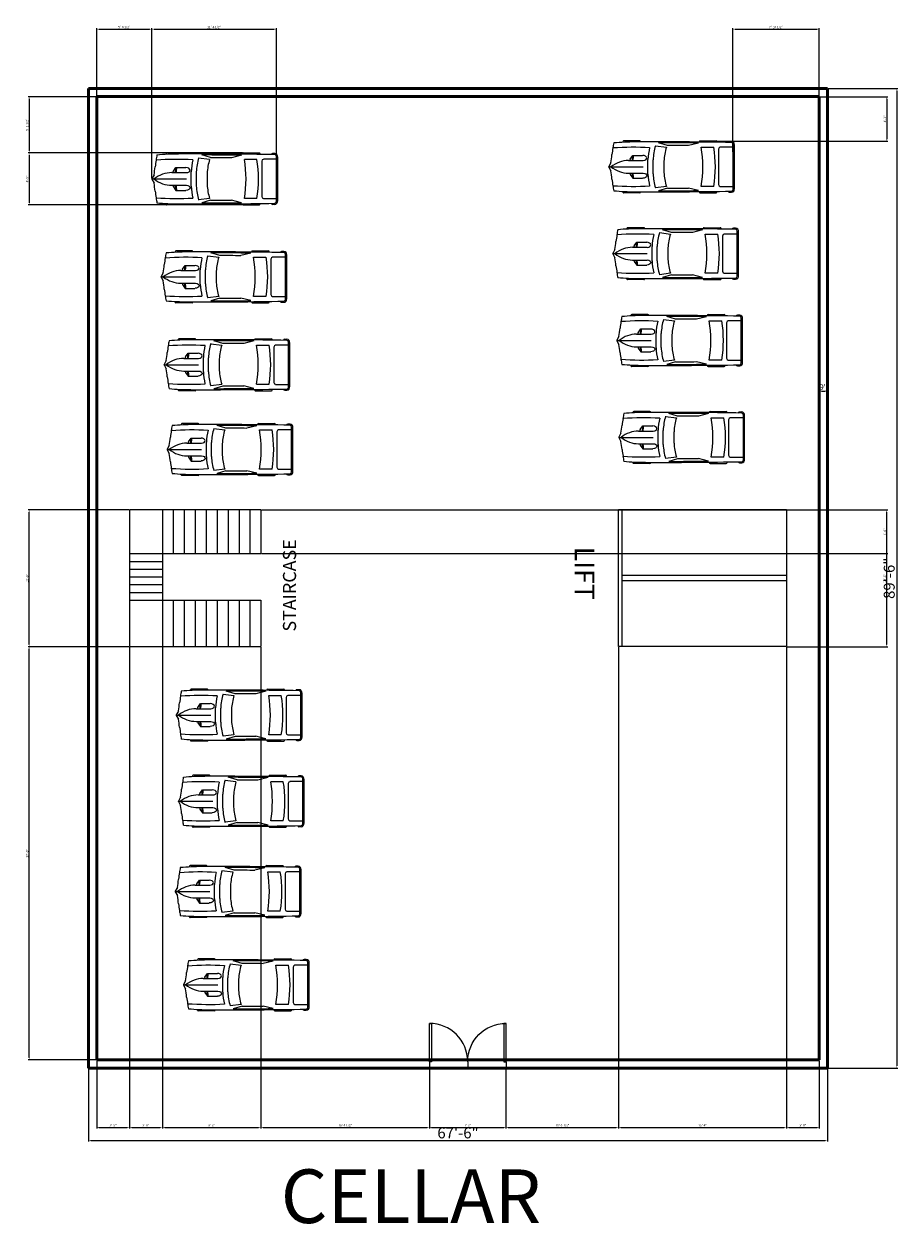
# Model space of a CAD drawing. Units: inches. Extents: x -12550 to 6516, y 1273 to 18700.
# Tile 1 of 19: x 757 to 1715, y 1273 to 2589. Entities that reach past the tile are written whole.
import ezdxf

# ---------------------------------------------------------------- set-up
doc = ezdxf.new("R2010")
doc.units = ezdxf.units.IN
for name, color, linetype, lineweight in [('A-ANNO-DIMS', 2, 'Continuous', 18), ('A-ANNO-TEXT', 7, 'Continuous', 25), ('A-AREA-IDEN', 1, 'Continuous', 18), ('A-DOOR', 5, 'Continuous', 25), ('A-EQPM', 4, 'Continuous', 25), ('A-FLOR-STRS', 6, 'Continuous', 25), ('A-FURN', 8, 'Continuous', 18), ('A-WALL', 7, 'Continuous', 50)]:
    doc.layers.add(name, color=color, linetype=linetype, lineweight=lineweight)
doc.styles.get("Standard").update_dxf_attribs({"font": 'arial.ttf'})
doc.dimstyles.new('ISO-25', dxfattribs={"dimtxt": 2.5, "dimasz": 2.5, "dimexe": 1.25, "dimexo": 0.625, "dimtad": 1, "dimlunit": 4, "dimtxsty": 'Standard', "dimcen": 2.5, "dimadec": 0, "dimazin": 0, "dimtfac": 1, "dimtmove": 0, "dimatfit": 3, "dimfxl": 1, "dimarcsym": 0})

# ---------------------------------------------------------------- blocks, each defined once
blk = doc.blocks.new('*U2')
for p, q in [((0, 0), (0, -5)), ((30, 0), (30, -5))]:
    blk.add_line(p, q)
blk.add_lwpolyline([(0, 0), (0, 30), (1.75, 30), (1.75, 0)], close=True)
blk.add_arc((0, 0), 30, 0, 90)
blk = doc.blocks.new('*D22')
at = {"layer": 'A-ANNO-DIMS', "color": 0, "lineweight": -2, "transparency": 16777216}
for p, q in [((1638, 2518.2), (1714.6, 2518.2)), ((1713.4, 2515.7), (1713.4, 1446.7)), ((1638, 1444.2), (1714.6, 1444.2))]:
    blk.add_line(p, q, dxfattribs=at)
at = {"layer": 'A-ANNO-DIMS', "color": 0, "transparency": 16777216}
for points in [[(1713, 2515.7), (1713.8, 2515.7), (1713.4, 2518.2)], [(1713, 1446.7), (1713.8, 1446.7), (1713.4, 1444.2)]]:
    blk.add_solid(points, dxfattribs=at)
at = {"layer": 'Defpoints', "color": 0, "transparency": 16777216}
for p in [(1637.4, 2518.2), (1637.4, 1444.2), (1713.4, 1444.2)]:
    blk.add_point(p, dxfattribs=at)
at = {"layer": 'A-ANNO-DIMS', "color": 0, "transparency": 16777216, "insert": (1706.6, 1981.2), "char_height": 12, "attachment_point": 5, "rotation": 90}
blk.add_mtext('89\'-6"', dxfattribs=at)
blk = doc.blocks.new('*D23')
at = {"layer": 'A-ANNO-DIMS', "color": 0, "lineweight": -2, "transparency": 16777216}
for p, q in [((827.4, 1443.6), (827.4, 1363.6)), ((1637.4, 1443.6), (1637.4, 1363.6)), ((829.9, 1364.9), (1634.9, 1364.9))]:
    blk.add_line(p, q, dxfattribs=at)
at = {"layer": 'A-ANNO-DIMS', "color": 0, "transparency": 16777216}
for points in [[(829.9, 1365.3), (829.9, 1364.5), (827.4, 1364.9)], [(1634.9, 1365.3), (1634.9, 1364.5), (1637.4, 1364.9)]]:
    blk.add_solid(points, dxfattribs=at)
at = {"layer": 'Defpoints', "color": 0, "transparency": 16777216}
for p in [(827.4, 1444.2), (1637.4, 1444.2), (1637.4, 1364.9)]:
    blk.add_point(p, dxfattribs=at)
at = {"layer": 'A-ANNO-DIMS', "color": 0, "transparency": 16777216, "insert": (1232.4, 1371.6), "char_height": 12, "attachment_point": 5}
blk.add_mtext('67\'-6"', dxfattribs=at)
blk = doc.blocks.new('*D24')
at = {"layer": 'A-ANNO-DIMS', "color": 0, "lineweight": -2, "transparency": 16777216}
for p, q in [((1628.4, 2172.1), (1628.4, 2187.7)), ((1630.9, 2186.4), (1634.9, 2186.4)), ((1637.4, 2172.1), (1637.4, 2187.7))]:
    blk.add_line(p, q, dxfattribs=at)
at = {"layer": 'A-ANNO-DIMS', "color": 0, "transparency": 16777216}
for points in [[(1630.9, 2186.9), (1630.9, 2186), (1628.4, 2186.4)], [(1634.9, 2186.9), (1634.9, 2186), (1637.4, 2186.4)]]:
    blk.add_solid(points, dxfattribs=at)
at = {"layer": 'Defpoints', "color": 0, "transparency": 16777216}
for p in [(1637.4, 2186.4), (1628.4, 2171.4), (1637.4, 2171.4)]:
    blk.add_point(p, dxfattribs=at)
at = {"layer": 'A-ANNO-DIMS', "color": 0, "transparency": 16777216, "insert": (1632.9, 2190.1), "char_height": 6, "attachment_point": 5}
blk.add_mtext('9"', dxfattribs=at)
blk = doc.blocks.new('*U21')
for p, q in [((21.1, 37.4), (21.1, 36.8)), ((46.6, 38.9), (22.4, 38.9)), ((47.8, 37.4), (47.8, 37.4)), ((135.5, 37.1), (135.5, 37.4)), ((136.7, 38.9), (160.9, 38.9)), ((162.1, 37.4), (162.1, 36.8)), ((70, 31.5), (86.4, 29.4)), ((88, 31.9), (74.8, 35.9)), ((134.3, 35.6), (119.3, 31.8)), ((138.4, 29.4), (157.2, 29.4)), ((164.5, 26.4), (164.5, -26.4)), ((186.5, 29.4), (167, 29.4)), ((186.5, -33.5), (186.5, 33.5)), ((188.4, -32.8), (188.4, 32.8)), ((3.3, 6.1), (0.1, 0.4)), ((29.8, 9.5), (51.7, 9.5)), ((32.1, 9.5), (32.1, 11.2)), ((32.3, 11.6), (36.1, 17.2)), ((36.1, 17.2), (50.9, 17.2)), ((58.9, -10.8), (58.9, 10.8)), ((66.6, -10.5), (66.6, 10.5)), ((82.7, 8.5), (82.7, -8.5)), ((186.5, -10.5), (186.5, 10.5)), ((0, 0), (51.7, 0)), ((0.1, -0.4), (3.3, -6.1)), ((29.8, -9.5), (51.7, -9.5)), ((32.1, -9.5), (32.1, -11.2)), ((32.3, -11.6), (36.1, -17.2)), ((36.1, -17.2), (50.9, -17.2)), ((86.4, -29.4), (70, -31.5)), ((88, -31.9), (74.8, -35.9)), ((134.3, -35.6), (119.3, -31.8)), ((157.2, -29.4), (138.4, -29.4)), ((167, -29.4), (186.5, -29.4)), ((21.1, -37.4), (21.1, -36.8)), ((46.6, -38.9), (22.4, -38.9)), ((47.8, -37.4), (47.8, -37.4)), ((135.5, -37.1), (135.5, -37.4)), ((136.7, -38.9), (160.9, -38.9)), ((162.1, -37.4), (162.1, -36.8))]:
    blk.add_line(p, q)
for centre, major_axis, ratio, start_param, end_param in [((41.2, -490.9), (0, 528.2), 0.842304, 0.00281, 0.075598), ((22.4, 37.4), (0, -1.48), 0.842304, 3.141593, 4.712389), ((64.5, -10555.6), (0, 10593), 0.842304, -0.013397, 0.002797), ((46.6, 37.4), (0, 1.48), 0.842304, -1.570796, 0), ((136.7, 37.4), (0, -1.48), 0.842304, 3.141593, 4.712389), ((160.9, 37.4), (0, 1.48), 0.842304, -1.570796, 0), ((180.6, 35.8), (0, 2.22), 0.842304, -0.013017, 1.249894), ((64.5, -10556.4), (0, 10595.3), 0.842304, -0.013397, -0.013017), ((184, 32.8), (0, -5.25), 0.842304, 1.570796, 3.128196), ((184, 33.5), (0, -2.96), 0.842304, 1.570796, 3.128196), ((-204.5, 52.4), (0, -251), 0.842304, 1.385369, 1.434372), ((259.2, -27.5), (0, -305.3), 0.842304, 4.528606, 4.561838), ((266, -27.5), (0, 313.3), 0.842304, 1.367076, 1.39176), ((37.5, -594), (0, -623.3), 0.842304, 3.096046, 3.200911), ((134.4, 5.4), (0, -89.8), 0.842304, 4.449482, 4.652344), ((135.3, 5.4), (0, 81.8), 0.842304, 1.245306, 1.50788), ((64.5, -10555.6), (0, -10591.5), 0.842304, 3.133765, 3.140441), ((149.6, 2.8), (0, -79.6), 0.842304, 4.372215, 4.640744), ((95.8, -3666.4), (0, -3698.2), 0.842304, 3.134049, 3.144098), ((17.1, 0), (0, 147), 0.842304, 4.511394, 4.913384), ((35.9, 0), (0, 147), 0.842304, 4.511394, 4.913384), ((167, 26.4), (0, 2.96), 0.842304, 0, 1.570796), ((0.6, 0), (0, -0.74), 0.842304, 4.131459, 5.293319), ((29.8, -46.7), (0, 56.2), 0.842304, 0, 0.590319), ((32.7, 11.2), (0, 0.74), 0.842304, 0.879714, 1.570796), ((13, 17), (0, 27.4), 0.842304, 4.435146, 4.718221), ((14.2, 17), (0, 27.4), 0.842304, 4.435146, 4.718221), ((50.8, 13.3), (6.34, -0.36), 0.603834, -1.395552, 1.581315), ((-204.5, -52.4), (0, 251), 0.842304, -1.434372, -1.385369), ((29.8, 46.7), (0, 56.2), 0.842304, 2.551274, 3.141593), ((32.7, -11.2), (0, -0.74), 0.842304, 4.712389, 5.403472), ((13, -17), (0, -27.4), 0.842304, 1.564964, 1.848039), ((14.2, -17), (0, -27.4), 0.842304, 1.564964, 1.848039), ((134.4, -5.4), (0, -89.8), 0.842304, -1.510751, -1.307889), ((135.3, -5.4), (0, -81.8), 0.842304, -1.50788, -1.245306), ((149.6, -2.8), (0, -79.6), 0.842304, -1.499151, -1.230623), ((259.2, 27.5), (0, 305.3), 0.842304, 1.721348, 1.754579), ((266, 27.5), (0, 313.3), 0.842304, 1.749832, 1.774517), ((37.5, 594), (0, -623.3), 0.842304, -0.059319, 0.045547), ((41.2, 490.9), (0, -528.2), 0.842304, -0.075598, -0.00281), ((64.5, 10555.6), (0, -10591.5), 0.842304, 0.001152, 0.007828), ((95.8, 3666.4), (0, -3698.2), 0.842304, -0.002505, 0.007544), ((167, -26.4), (0, -2.96), 0.842304, 4.712389, 6.283185), ((184, -32.8), (0, -5.25), 0.842304, 0.013397, 1.570796), ((184, -33.5), (0, 2.96), 0.842304, 3.15499, 4.712389), ((22.4, -37.4), (0, 1.48), 0.842304, 1.570796, 3.141593), ((64.5, 10555.6), (0, 10593), 0.842304, 3.138796, 3.15499), ((46.6, -37.4), (0, -1.48), 0.842304, 0, 1.570796), ((136.7, -37.4), (0, -1.48), 0.842304, -1.570796, 0), ((160.9, -37.4), (0, 1.48), 0.842304, 3.141593, 4.712389), ((180.6, -35.8), (0, -2.22), 0.842304, -1.249894, 0.013017), ((64.5, 10556.4), (0, 10595.3), 0.842304, 3.15461, 3.15499)]:
    blk.add_ellipse(centre, major_axis=major_axis, ratio=ratio, start_param=start_param, end_param=end_param)
at = {"extrusion": (0, 0, -1)}
blk.add_ellipse((50.8, -13.3), major_axis=(6.34, 0.36), ratio=0.603834, start_param=-1.395552, end_param=1.581315, dxfattribs=at)
blk = doc.blocks.new('*D77')
at = {"layer": 'A-ANNO-DIMS', "color": 0, "lineweight": -2, "transparency": 16777216}
for p, q in [((872.4, 1905.6), (872.4, 1378)), ((836.4, 1452.6), (836.4, 1378)), ((838.9, 1379.2), (869.9, 1379.2))]:
    blk.add_line(p, q, dxfattribs=at)
at = {"layer": 'A-ANNO-DIMS', "color": 0, "transparency": 16777216}
for points in [[(838.9, 1379.7), (838.9, 1378.8), (836.4, 1379.2)], [(869.9, 1379.7), (869.9, 1378.8), (872.4, 1379.2)]]:
    blk.add_solid(points, dxfattribs=at)
at = {"layer": 'Defpoints', "color": 0, "transparency": 16777216}
for p in [(872.4, 1906.2), (836.4, 1453.2), (872.4, 1379.2)]:
    blk.add_point(p, dxfattribs=at)
at = {"layer": 'A-ANNO-DIMS', "color": 0, "transparency": 16777216, "insert": (854.4, 1381.1), "char_height": 2.5, "attachment_point": 5}
blk.add_mtext('3\'-0"', dxfattribs=at)
blk = doc.blocks.new('*D78')
at = {"layer": 'A-ANNO-DIMS', "color": 0, "lineweight": -2, "transparency": 16777216}
for p, q in [((872.4, 1905.6), (872.4, 1378)), ((908.4, 1905.6), (908.4, 1378)), ((874.9, 1379.2), (905.9, 1379.2))]:
    blk.add_line(p, q, dxfattribs=at)
at = {"layer": 'A-ANNO-DIMS', "color": 0, "transparency": 16777216}
for points in [[(874.9, 1379.7), (874.9, 1378.8), (872.4, 1379.2)], [(905.9, 1379.7), (905.9, 1378.8), (908.4, 1379.2)]]:
    blk.add_solid(points, dxfattribs=at)
at = {"layer": 'Defpoints', "color": 0, "transparency": 16777216}
for p in [(872.4, 1906.2), (908.4, 1906.2), (908.4, 1379.2)]:
    blk.add_point(p, dxfattribs=at)
at = {"layer": 'A-ANNO-DIMS', "color": 0, "transparency": 16777216, "insert": (890.4, 1381.1), "char_height": 2.5, "attachment_point": 5}
blk.add_mtext('3\'-0"', dxfattribs=at)
blk = doc.blocks.new('*D79')
at = {"layer": 'A-ANNO-DIMS', "color": 0, "lineweight": -2, "transparency": 16777216}
for p, q in [((908.4, 1905.6), (908.4, 1378)), ((1016.4, 1905.6), (1016.4, 1378)), ((910.9, 1379.2), (1013.9, 1379.2))]:
    blk.add_line(p, q, dxfattribs=at)
at = {"layer": 'A-ANNO-DIMS', "color": 0, "transparency": 16777216}
for points in [[(910.9, 1379.7), (910.9, 1378.8), (908.4, 1379.2)], [(1013.9, 1379.7), (1013.9, 1378.8), (1016.4, 1379.2)]]:
    blk.add_solid(points, dxfattribs=at)
at = {"layer": 'Defpoints', "color": 0, "transparency": 16777216}
for p in [(908.4, 1906.2), (1016.4, 1906.2), (1016.4, 1379.2)]:
    blk.add_point(p, dxfattribs=at)
at = {"layer": 'A-ANNO-DIMS', "color": 0, "transparency": 16777216, "insert": (962.4, 1381.1), "char_height": 2.5, "attachment_point": 5}
blk.add_mtext('9\'-0"', dxfattribs=at)
blk = doc.blocks.new('*D80')
at = {"layer": 'A-ANNO-DIMS', "color": 0, "lineweight": -2, "transparency": 16777216}
for p, q in [((1016.4, 1905.6), (1016.4, 1378)), ((1201, 1443.6), (1201, 1378)), ((1018.9, 1379.2), (1198.5, 1379.2))]:
    blk.add_line(p, q, dxfattribs=at)
at = {"layer": 'A-ANNO-DIMS', "color": 0, "transparency": 16777216}
for points in [[(1018.9, 1379.7), (1018.9, 1378.8), (1016.4, 1379.2)], [(1198.5, 1379.7), (1198.5, 1378.8), (1201, 1379.2)]]:
    blk.add_solid(points, dxfattribs=at)
at = {"layer": 'Defpoints', "color": 0, "transparency": 16777216}
for p in [(1016.4, 1906.2), (1201, 1444.2), (1201, 1379.2)]:
    blk.add_point(p, dxfattribs=at)
at = {"layer": 'A-ANNO-DIMS', "color": 0, "transparency": 16777216, "insert": (1108.7, 1381.2), "char_height": 2.5, "attachment_point": 5}
blk.add_mtext('15\'-4 1/2"', dxfattribs=at)
blk = doc.blocks.new('*D81')
at = {"layer": 'A-ANNO-DIMS', "color": 0, "lineweight": -2, "transparency": 16777216}
for p, q in [((1201, 1443.6), (1201, 1378)), ((1285, 1443.6), (1285, 1378)), ((1203.5, 1379.2), (1282.5, 1379.2))]:
    blk.add_line(p, q, dxfattribs=at)
at = {"layer": 'A-ANNO-DIMS', "color": 0, "transparency": 16777216}
for points in [[(1203.5, 1379.7), (1203.5, 1378.8), (1201, 1379.2)], [(1282.5, 1379.7), (1282.5, 1378.8), (1285, 1379.2)]]:
    blk.add_solid(points, dxfattribs=at)
at = {"layer": 'Defpoints', "color": 0, "transparency": 16777216}
for p in [(1201, 1444.2), (1285, 1444.2), (1285, 1379.2)]:
    blk.add_point(p, dxfattribs=at)
at = {"layer": 'A-ANNO-DIMS', "color": 0, "transparency": 16777216, "insert": (1243, 1381.1), "char_height": 2.5, "attachment_point": 5}
blk.add_mtext('7\'-0"', dxfattribs=at)
blk = doc.blocks.new('*D82')
at = {"layer": 'A-ANNO-DIMS', "color": 0, "lineweight": -2, "transparency": 16777216}
for p, q in [((1408.4, 1905.6), (1408.4, 1378)), ((1285, 1443.6), (1285, 1378)), ((1287.5, 1379.2), (1405.9, 1379.2))]:
    blk.add_line(p, q, dxfattribs=at)
at = {"layer": 'A-ANNO-DIMS', "color": 0, "transparency": 16777216}
for points in [[(1287.5, 1379.7), (1287.5, 1378.8), (1285, 1379.2)], [(1405.9, 1379.7), (1405.9, 1378.8), (1408.4, 1379.2)]]:
    blk.add_solid(points, dxfattribs=at)
at = {"layer": 'Defpoints', "color": 0, "transparency": 16777216}
for p in [(1408.4, 1906.2), (1285, 1444.2), (1408.4, 1379.2)]:
    blk.add_point(p, dxfattribs=at)
at = {"layer": 'A-ANNO-DIMS', "color": 0, "transparency": 16777216, "insert": (1346.7, 1381.2), "char_height": 2.5, "attachment_point": 5}
blk.add_mtext('10\'-3 1/2"', dxfattribs=at)
blk = doc.blocks.new('*D83')
at = {"layer": 'A-ANNO-DIMS', "color": 0, "lineweight": -2, "transparency": 16777216}
for p, q in [((1408.4, 1905.6), (1408.4, 1378)), ((1592.4, 1905.6), (1592.4, 1378)), ((1410.9, 1379.2), (1589.9, 1379.2))]:
    blk.add_line(p, q, dxfattribs=at)
at = {"layer": 'A-ANNO-DIMS', "color": 0, "transparency": 16777216}
for points in [[(1410.9, 1379.7), (1410.9, 1378.8), (1408.4, 1379.2)], [(1589.9, 1379.7), (1589.9, 1378.8), (1592.4, 1379.2)]]:
    blk.add_solid(points, dxfattribs=at)
at = {"layer": 'Defpoints', "color": 0, "transparency": 16777216}
for p in [(1408.4, 1906.2), (1592.4, 1906.2), (1592.4, 1379.2)]:
    blk.add_point(p, dxfattribs=at)
at = {"layer": 'A-ANNO-DIMS', "color": 0, "transparency": 16777216, "insert": (1500.4, 1381.1), "char_height": 2.5, "attachment_point": 5}
blk.add_mtext('15\'-4"', dxfattribs=at)
blk = doc.blocks.new('*D84')
at = {"layer": 'A-ANNO-DIMS', "color": 0, "lineweight": -2, "transparency": 16777216}
for p, q in [((1592.4, 1905.6), (1592.4, 1378)), ((1628.4, 1452.6), (1628.4, 1378)), ((1594.9, 1379.2), (1625.9, 1379.2))]:
    blk.add_line(p, q, dxfattribs=at)
at = {"layer": 'A-ANNO-DIMS', "color": 0, "transparency": 16777216}
for points in [[(1594.9, 1379.7), (1594.9, 1378.8), (1592.4, 1379.2)], [(1625.9, 1379.7), (1625.9, 1378.8), (1628.4, 1379.2)]]:
    blk.add_solid(points, dxfattribs=at)
at = {"layer": 'Defpoints', "color": 0, "transparency": 16777216}
for p in [(1592.4, 1906.2), (1628.4, 1453.2), (1628.4, 1379.2)]:
    blk.add_point(p, dxfattribs=at)
at = {"layer": 'A-ANNO-DIMS', "color": 0, "transparency": 16777216, "insert": (1610.4, 1381.1), "char_height": 2.5, "attachment_point": 5}
blk.add_mtext('3\'-0"', dxfattribs=at)
blk = doc.blocks.new('*D85')
at = {"layer": 'A-ANNO-DIMS', "color": 0, "lineweight": -2, "transparency": 16777216}
for p, q in [((871.7, 2056.2), (761.1, 2056.2)), ((762.4, 1908.7), (762.4, 2053.7)), ((871.7, 1906.2), (761.1, 1906.2))]:
    blk.add_line(p, q, dxfattribs=at)
at = {"layer": 'A-ANNO-DIMS', "color": 0, "transparency": 16777216}
for points in [[(761.9, 2053.7), (762.8, 2053.7), (762.4, 2056.2)], [(761.9, 1908.7), (762.8, 1908.7), (762.4, 1906.2)]]:
    blk.add_solid(points, dxfattribs=at)
at = {"layer": 'Defpoints', "color": 0, "transparency": 16777216}
for p in [(762.4, 2056.2), (872.4, 2056.2), (872.4, 1906.2)]:
    blk.add_point(p, dxfattribs=at)
at = {"layer": 'A-ANNO-DIMS', "color": 0, "transparency": 16777216, "insert": (760.5, 1981.2), "char_height": 2.5, "attachment_point": 5, "rotation": 90}
blk.add_mtext('12\'-6"', dxfattribs=at)
blk = doc.blocks.new('*D86')
at = {"layer": 'A-ANNO-DIMS', "color": 0, "lineweight": -2, "transparency": 16777216}
for p, q in [((871.7, 1906.2), (761.1, 1906.2)), ((762.4, 1455.7), (762.4, 1903.7)), ((835.7, 1453.2), (761.1, 1453.2))]:
    blk.add_line(p, q, dxfattribs=at)
at = {"layer": 'A-ANNO-DIMS', "color": 0, "transparency": 16777216}
for points in [[(761.9, 1903.7), (762.8, 1903.7), (762.4, 1906.2)], [(761.9, 1455.7), (762.8, 1455.7), (762.4, 1453.2)]]:
    blk.add_solid(points, dxfattribs=at)
at = {"layer": 'Defpoints', "color": 0, "transparency": 16777216}
for p in [(762.4, 1906.2), (872.4, 1906.2), (836.4, 1453.2)]:
    blk.add_point(p, dxfattribs=at)
at = {"layer": 'A-ANNO-DIMS', "color": 0, "transparency": 16777216, "insert": (760.5, 1679.7), "char_height": 2.5, "attachment_point": 5, "rotation": 90}
blk.add_mtext('37\'-9"', dxfattribs=at)
blk = doc.blocks.new('*D87')
at = {"layer": 'A-ANNO-DIMS', "color": 0, "lineweight": -2, "transparency": 16777216}
for p, q in [((1017, 2056.2), (1703.6, 2056.2)), ((1702.4, 2010.7), (1702.4, 2053.7)), ((1017, 2008.2), (1703.6, 2008.2))]:
    blk.add_line(p, q, dxfattribs=at)
at = {"layer": 'A-ANNO-DIMS', "color": 0, "transparency": 16777216}
for points in [[(1701.9, 2053.7), (1702.8, 2053.7), (1702.4, 2056.2)], [(1701.9, 2010.7), (1702.8, 2010.7), (1702.4, 2008.2)]]:
    blk.add_solid(points, dxfattribs=at)
at = {"layer": 'Defpoints', "color": 0, "transparency": 16777216}
for p in [(1016.4, 2056.2), (1702.4, 2056.2), (1016.4, 2008.2)]:
    blk.add_point(p, dxfattribs=at)
at = {"layer": 'A-ANNO-DIMS', "color": 0, "transparency": 16777216, "insert": (1700.5, 2032.2), "char_height": 2.5, "attachment_point": 5, "rotation": 90}
blk.add_mtext('4\'-0"', dxfattribs=at)
blk = doc.blocks.new('*D88')
at = {"layer": 'A-ANNO-DIMS', "color": 0, "lineweight": -2, "transparency": 16777216}
for p, q in [((1593, 2056.2), (1703.6, 2056.2)), ((1702.4, 1908.7), (1702.4, 2053.7)), ((1593, 1906.2), (1703.6, 1906.2))]:
    blk.add_line(p, q, dxfattribs=at)
at = {"layer": 'A-ANNO-DIMS', "color": 0, "transparency": 16777216}
for points in [[(1701.9, 2053.7), (1702.8, 2053.7), (1702.4, 2056.2)], [(1701.9, 1908.7), (1702.8, 1908.7), (1702.4, 1906.2)]]:
    blk.add_solid(points, dxfattribs=at)
at = {"layer": 'Defpoints', "color": 0, "transparency": 16777216}
for p in [(1592.4, 2056.2), (1702.4, 2056.2), (1592.4, 1906.2)]:
    blk.add_point(p, dxfattribs=at)
at = {"layer": 'A-ANNO-DIMS', "color": 0, "transparency": 16777216, "insert": (1700.5, 1981.2), "char_height": 2.5, "attachment_point": 5, "rotation": 90}
blk.add_mtext('12\'-6"', dxfattribs=at)
blk = doc.blocks.new('*D89')
at = {"layer": 'A-ANNO-DIMS', "color": 0, "lineweight": -2, "transparency": 16777216}
for p, q in [((896.9, 2419.8), (896.9, 2584.5)), ((899.4, 2583.2), (1030.8, 2583.2)), ((1033.3, 2435.6), (1033.3, 2584.5))]:
    blk.add_line(p, q, dxfattribs=at)
at = {"layer": 'A-ANNO-DIMS', "color": 0, "transparency": 16777216}
for points in [[(899.4, 2583.7), (899.4, 2582.8), (896.9, 2583.2)], [(1030.8, 2583.7), (1030.8, 2582.8), (1033.3, 2583.2)]]:
    blk.add_solid(points, dxfattribs=at)
at = {"layer": 'Defpoints', "color": 0, "transparency": 16777216}
for p in [(1033.3, 2583.2), (1033.3, 2435), (896.9, 2419.2)]:
    blk.add_point(p, dxfattribs=at)
at = {"layer": 'A-ANNO-DIMS', "color": 0, "transparency": 16777216, "insert": (965.1, 2585.2), "char_height": 2.5, "attachment_point": 5}
blk.add_mtext('11\'-4 1/2"', dxfattribs=at)
blk = doc.blocks.new('*D90')
at = {"layer": 'A-ANNO-DIMS', "color": 0, "lineweight": -2, "transparency": 16777216}
for p, q in [((996.3, 2447.5), (761.1, 2447.5)), ((762.4, 2445), (762.4, 2393)), ((996.3, 2390.5), (761.1, 2390.5))]:
    blk.add_line(p, q, dxfattribs=at)
at = {"layer": 'A-ANNO-DIMS', "color": 0, "transparency": 16777216}
for points in [[(761.9, 2445), (762.8, 2445), (762.4, 2447.5)], [(761.9, 2393), (762.8, 2393), (762.4, 2390.5)]]:
    blk.add_solid(points, dxfattribs=at)
at = {"layer": 'Defpoints', "color": 0, "transparency": 16777216}
for p in [(997, 2447.5), (762.4, 2390.5), (997, 2390.5)]:
    blk.add_point(p, dxfattribs=at)
at = {"layer": 'A-ANNO-DIMS', "color": 0, "transparency": 16777216, "insert": (760.5, 2419), "char_height": 2.5, "attachment_point": 5, "rotation": 90}
blk.add_mtext('4\'-9"', dxfattribs=at)
blk = doc.blocks.new('*D91')
at = {"layer": 'A-ANNO-DIMS', "color": 0, "lineweight": -2, "transparency": 16777216}
for p, q in [((836.4, 2509.9), (836.4, 2584.5)), ((838.9, 2583.2), (894.4, 2583.2)), ((896.9, 2419.8), (896.9, 2584.5))]:
    blk.add_line(p, q, dxfattribs=at)
at = {"layer": 'A-ANNO-DIMS', "color": 0, "transparency": 16777216}
for points in [[(838.9, 2583.7), (838.9, 2582.8), (836.4, 2583.2)], [(894.4, 2583.7), (894.4, 2582.8), (896.9, 2583.2)]]:
    blk.add_solid(points, dxfattribs=at)
at = {"layer": 'Defpoints', "color": 0, "transparency": 16777216}
for p in [(896.9, 2583.2), (836.4, 2509.2), (896.9, 2419.2)]:
    blk.add_point(p, dxfattribs=at)
at = {"layer": 'A-ANNO-DIMS', "color": 0, "transparency": 16777216, "insert": (866.6, 2585.2), "char_height": 2.5, "attachment_point": 5}
blk.add_mtext('5\'-0 1/2"', dxfattribs=at)
blk = doc.blocks.new('*D92')
at = {"layer": 'A-ANNO-DIMS', "color": 0, "lineweight": -2, "transparency": 16777216}
for p, q in [((835.7, 2509.2), (761.1, 2509.2)), ((762.4, 2506.7), (762.4, 2450.2)), ((923.6, 2447.7), (761.1, 2447.7))]:
    blk.add_line(p, q, dxfattribs=at)
at = {"layer": 'A-ANNO-DIMS', "color": 0, "transparency": 16777216}
for points in [[(761.9, 2506.7), (762.8, 2506.7), (762.4, 2509.2)], [(761.9, 2450.2), (762.8, 2450.2), (762.4, 2447.7)]]:
    blk.add_solid(points, dxfattribs=at)
at = {"layer": 'Defpoints', "color": 0, "transparency": 16777216}
for p in [(836.4, 2509.2), (762.4, 2447.7), (924.2, 2447.7)]:
    blk.add_point(p, dxfattribs=at)
at = {"layer": 'A-ANNO-DIMS', "color": 0, "transparency": 16777216, "insert": (760.4, 2478.5), "char_height": 2.5, "attachment_point": 5, "rotation": 90}
blk.add_mtext('5\'-1 1/2"', dxfattribs=at)
blk = doc.blocks.new('*D93')
at = {"layer": 'A-ANNO-DIMS', "color": 0, "lineweight": -2, "transparency": 16777216}
for p, q in [((1533.6, 2448.7), (1533.6, 2584.5)), ((1536.1, 2583.2), (1625.9, 2583.2)), ((1628.4, 2509.9), (1628.4, 2584.5))]:
    blk.add_line(p, q, dxfattribs=at)
at = {"layer": 'A-ANNO-DIMS', "color": 0, "transparency": 16777216}
for points in [[(1536.1, 2583.7), (1536.1, 2582.8), (1533.6, 2583.2)], [(1625.9, 2583.7), (1625.9, 2582.8), (1628.4, 2583.2)]]:
    blk.add_solid(points, dxfattribs=at)
at = {"layer": 'Defpoints', "color": 0, "transparency": 16777216}
for p in [(1628.4, 2583.2), (1628.4, 2509.2), (1533.6, 2448.1)]:
    blk.add_point(p, dxfattribs=at)
at = {"layer": 'A-ANNO-DIMS', "color": 0, "transparency": 16777216, "insert": (1581, 2585.2), "char_height": 2.5, "attachment_point": 5}
blk.add_mtext('7\'-10 1/2"', dxfattribs=at)
blk = doc.blocks.new('*D94')
at = {"layer": 'A-ANNO-DIMS', "color": 0, "lineweight": -2, "transparency": 16777216}
for p, q in [((1629, 2509.2), (1703.6, 2509.2)), ((1702.4, 2506.7), (1702.4, 2462.8)), ((1500.9, 2460.3), (1703.6, 2460.3))]:
    blk.add_line(p, q, dxfattribs=at)
at = {"layer": 'A-ANNO-DIMS', "color": 0, "transparency": 16777216}
for points in [[(1701.9, 2506.7), (1702.8, 2506.7), (1702.4, 2509.2)], [(1701.9, 2462.8), (1702.8, 2462.8), (1702.4, 2460.3)]]:
    blk.add_solid(points, dxfattribs=at)
at = {"layer": 'Defpoints', "color": 0, "transparency": 16777216}
for p in [(1628.4, 2509.2), (1500.2, 2460.3), (1702.4, 2460.3)]:
    blk.add_point(p, dxfattribs=at)
at = {"layer": 'A-ANNO-DIMS', "color": 0, "transparency": 16777216, "insert": (1700.5, 2484.8), "char_height": 2.5, "attachment_point": 5, "rotation": 90}
blk.add_mtext('4\'-1"', dxfattribs=at)

msp = doc.modelspace()

# ---------------------------------------------------------------- linework, layer by layer
at = {"layer": 'A-EQPM'}
for p, q in [((1408.361, 1906.247), (1408.361, 2056.247)), ((1592.361, 2056.247), (1408.361, 2056.247)), ((1412.361, 1906.247), (1412.361, 2056.247)), ((1592.361, 2056.247), (1592.361, 1906.247)), ((1592.361, 1984.247), (1412.361, 1984.247)), ((1592.361, 1978.247), (1412.361, 1978.247)), ((1592.361, 1906.247), (1408.361, 1906.247))]:
    msp.add_line(p, q, dxfattribs=at)
at = {"layer": 'A-FLOR-STRS'}
for p, q in [((1016.361, 2056.247), (872.361, 2056.247)), ((872.361, 2056.247), (872.361, 1906.247)), ((908.361, 2056.247), (908.361, 1906.247)), ((920.361, 2056.247), (920.361, 2008.247)), ((932.361, 2056.247), (932.361, 2008.247)), ((944.361, 2056.247), (944.361, 2008.247)), ((956.361, 2056.247), (956.361, 2008.247)), ((968.361, 2056.247), (968.361, 2008.247)), ((980.361, 2056.247), (980.361, 2008.247)), ((992.361, 2056.247), (992.361, 2008.247)), ((1004.361, 2056.247), (1004.361, 2008.247)), ((1016.361, 2056.247), (1016.361, 2008.247)), ((872.361, 2008.247), (1016.361, 2008.247)), ((872.361, 2008.247), (1016.361, 2008.247)), ((872.361, 1999.747), (908.361, 1999.747)), ((872.361, 1991.247), (908.361, 1991.247)), ((872.361, 1982.747), (908.361, 1982.747)), ((872.361, 1974.247), (908.361, 1974.247)), ((872.361, 1965.747), (908.361, 1965.747)), ((872.361, 1957.247), (1016.361, 1957.247)), ((920.361, 1957.247), (920.361, 1906.247)), ((932.361, 1957.247), (932.361, 1906.247)), ((944.361, 1957.247), (944.361, 1906.247)), ((956.361, 1957.247), (956.361, 1906.247)), ((968.361, 1957.247), (968.361, 1906.247)), ((980.361, 1957.247), (980.361, 1906.247)), ((992.361, 1957.247), (992.361, 1906.247)), ((1004.361, 1957.247), (1004.361, 1906.247)), ((1016.361, 1957.247), (1016.361, 1906.247)), ((872.361, 1906.247), (1016.361, 1906.247))]:
    msp.add_line(p, q, dxfattribs=at)
at = {"layer": 'A-WALL'}
for p, q in [((827.361, 1444.247), (827.361, 2518.247)), ((827.361, 2518.247), (1637.361, 2518.247)), ((1637.361, 2518.247), (1637.361, 1444.247)), ((836.361, 1453.247), (836.361, 2509.247)), ((836.361, 2509.247), (1628.361, 2509.247)), ((1628.361, 2509.247), (1628.361, 1453.247)), ((1628.361, 1489.247), (1628.361, 2060.923)), ((836.361, 1453.247), (1628.361, 1453.247)), ((827.361, 1444.247), (1637.361, 1444.247))]:
    msp.add_line(p, q, dxfattribs=at)

# ---------------------------------------------------------------- block references
at = {"layer": 'A-DOOR', "yscale": 1.399999999999999, "zscale": 1.399999999999999}
for p, xscale in [((1201.029, 1451.247), 1.399999999999999), ((1285.029, 1451.247), -1.399999999999999)]:
    msp.add_blockref('*U2', p, dxfattribs=dict(at, xscale=xscale))
at = {"layer": 'A-FURN', "xscale": 0.7323108405925999, "yscale": 0.7323108405925999, "zscale": 0.7323108405925999}
for p in [(1397.497, 2432.294), (896.857, 2419.012), (1401.928, 2337.107), (906.826, 2311.65), (1406.358, 2241.921), (910.149, 2215.357), (1408.573, 2135.666), (913.472, 2122.384), (923.573, 1831.225), (925.798, 1736.719), (922.461, 1637.766), (931.362, 1535.477)]:
    msp.add_blockref('*U21', p, dxfattribs=at)

# ---------------------------------------------------------------- texts
at = {"layer": 'A-ANNO-TEXT', "insert": (1038.16, 1333.138), "char_height": 58.816, "attachment_point": 1}
msp.add_mtext('CELLAR', dxfattribs=at)
at = {"layer": 'A-AREA-IDEN', "attachment_point": 1}
for s, width, gutter_width, insert, char_height, rotation in [('STAIRCASE', 2.19144, 71.795, (1040.538, 1922.837), 14.3589, 90), ('LIFT', 3.27433, 107.272, (1381.849, 2015.823), 21.4543, 270)]:
    msp.add_mtext_dynamic_manual_height_columns(s, width=width, gutter_width=gutter_width, heights=[0], dxfattribs=dict(at, insert=insert, char_height=char_height, rotation=rotation))

# ---------------------------------------------------------------- dimensions: what is measured, and where the dimension line sits
at = {"layer": 'A-ANNO-DIMS'}
for base, p1, p2, override, picture, middle in [((896.876, 2583.247), (836.361, 2509.247), (896.876, 2419.165), {"dimdec": 1, "dimlfac": 1, "dimrnd": 0, "dimzin": 1, "dimdsep": 46, "dimlunit": 4, "dimfrac": 2}, '*D91', (866.618, 2585.165)), ((1033.296, 2583.247), (896.876, 2419.165), (1033.296, 2434.984), {"dimdec": 1, "dimlfac": 1, "dimrnd": 0, "dimzin": 1, "dimdsep": 46, "dimlunit": 4, "dimfrac": 2}, '*D89', (965.086, 2585.165)), ((1628.361, 2583.247), (1533.625, 2448.067), (1628.361, 2509.247), {"dimdec": 1, "dimlfac": 1, "dimrnd": 0, "dimzin": 1, "dimdsep": 46, "dimlunit": 4, "dimfrac": 2}, '*D93', (1580.993, 2585.165)), ((1637.361, 2186.441), (1628.361, 2171.44), (1637.361, 2171.44), {"dimtxt": 6, "dimclrd": 0, "dimclre": 0, "dimclrt": 0}, '*D24', (1632.861, 2190.13)), ((872.361, 1379.247), (836.361, 1453.247), (872.361, 1906.247), {"dimdec": 1, "dimlfac": 1, "dimrnd": 0, "dimzin": 1, "dimdsep": 46, "dimlunit": 4, "dimfrac": 2}, '*D77', (854.361, 1381.15)), ((908.361, 1379.247), (872.361, 1906.247), (908.361, 1906.247), {"dimdec": 1, "dimlfac": 1, "dimrnd": 0, "dimzin": 1, "dimdsep": 46, "dimlunit": 4, "dimfrac": 2}, '*D78', (890.361, 1381.15)), ((1016.361, 1379.247), (908.361, 1906.247), (1016.361, 1906.247), {"dimdec": 1, "dimlfac": 1, "dimrnd": 0, "dimzin": 1, "dimdsep": 46, "dimlunit": 4, "dimfrac": 2}, '*D79', (962.361, 1381.149)), ((1201.029, 1379.247), (1016.361, 1906.247), (1201.029, 1444.247), {"dimdec": 1, "dimlfac": 1, "dimrnd": 0, "dimzin": 1, "dimdsep": 46, "dimlunit": 4, "dimfrac": 2}, '*D80', (1108.695, 1381.165)), ((1408.361, 1379.247), (1285.029, 1444.247), (1408.361, 1906.247), {"dimdec": 1, "dimlfac": 1, "dimrnd": 0, "dimzin": 1, "dimdsep": 46, "dimlunit": 4, "dimfrac": 2}, '*D82', (1346.695, 1381.166)), ((1592.361, 1379.247), (1408.361, 1906.247), (1592.361, 1906.247), {"dimdec": 1, "dimlfac": 1, "dimrnd": 0, "dimzin": 1, "dimdsep": 46, "dimlunit": 4, "dimfrac": 2}, '*D83', (1500.361, 1381.149)), ((1628.361, 1379.247), (1592.361, 1906.247), (1628.361, 1453.247), {"dimdec": 1, "dimlfac": 1, "dimrnd": 0, "dimzin": 1, "dimdsep": 46, "dimlunit": 4, "dimfrac": 2}, '*D84', (1610.361, 1381.15)), ((1637.361, 1364.887), (827.361, 1444.247), (1637.361, 1444.247), {"dimtxt": 12, "dimclrd": 0, "dimclre": 0, "dimclrt": 0}, '*D23', (1232.361, 1371.639)), ((1285.029, 1379.247), (1201.029, 1444.247), (1285.029, 1444.247), {"dimdec": 1, "dimlfac": 1, "dimrnd": 0, "dimzin": 1, "dimdsep": 46, "dimlunit": 4, "dimfrac": 2}, '*D81', (1243.029, 1381.149))]:
    dim = msp.add_linear_dim(base=base, p1=p1, p2=p2, dimstyle='ISO-25', override=override, dxfattribs=at)
    dim.commit()
    dim.dimension.update_dxf_attribs({"geometry": picture, "text_midpoint": middle})
for base, p1, p2, override, picture, middle in [((1713.396, 1444.247), (1637.361, 2518.247), (1637.361, 1444.247), {"dimtxt": 12, "dimclrd": 0, "dimclre": 0, "dimclrt": 0}, '*D22', (1706.644, 1981.247)), ((762.361, 2447.662), (836.361, 2509.247), (924.222, 2447.662), {"dimdec": 1, "dimlfac": 1, "dimrnd": 0, "dimzin": 1, "dimdsep": 46, "dimlunit": 4, "dimfrac": 2}, '*D92', (760.443, 2478.455)), ((1702.361, 2460.345), (1628.361, 2509.247), (1500.233, 2460.345), {"dimdec": 1, "dimlfac": 1, "dimrnd": 0, "dimzin": 1, "dimdsep": 46, "dimlunit": 4, "dimfrac": 2}, '*D94', (1700.481, 2484.796)), ((762.361, 2390.533), (996.963, 2447.49), (996.963, 2390.533), {"dimdec": 1, "dimlfac": 1, "dimrnd": 0, "dimzin": 1, "dimdsep": 46, "dimlunit": 4, "dimfrac": 2}, '*D90', (760.459, 2419.012)), ((762.361, 2056.247), (872.361, 1906.247), (872.361, 2056.247), {"dimdec": 1, "dimlfac": 1, "dimrnd": 0, "dimzin": 1, "dimdsep": 46, "dimlunit": 4, "dimfrac": 2}, '*D85', (760.459, 1981.247)), ((1702.361, 2056.247), (1016.361, 2008.247), (1016.361, 2056.247), {"dimdec": 1, "dimlfac": 1, "dimrnd": 0, "dimzin": 1, "dimdsep": 46, "dimlunit": 4, "dimfrac": 2}, '*D87', (1700.459, 2032.247)), ((1702.361, 2056.247), (1592.361, 1906.247), (1592.361, 2056.247), {"dimdec": 1, "dimlfac": 1, "dimrnd": 0, "dimzin": 1, "dimdsep": 46, "dimlunit": 4, "dimfrac": 2}, '*D88', (1700.459, 1981.247)), ((762.361, 1906.247), (836.361, 1453.247), (872.361, 1906.247), {"dimdec": 1, "dimlfac": 1, "dimrnd": 0, "dimzin": 1, "dimdsep": 46, "dimlunit": 4, "dimfrac": 2}, '*D86', (760.459, 1679.747))]:
    dim = msp.add_linear_dim(base=base, p1=p1, p2=p2, angle=90, dimstyle='ISO-25', override=override, dxfattribs=at)
    dim.commit()
    dim.dimension.update_dxf_attribs({"geometry": picture, "text_midpoint": middle})

doc.saveas('drawing.dxf')
